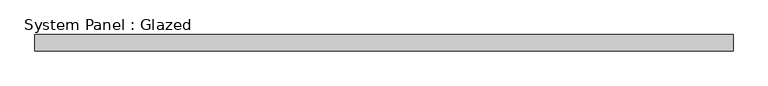
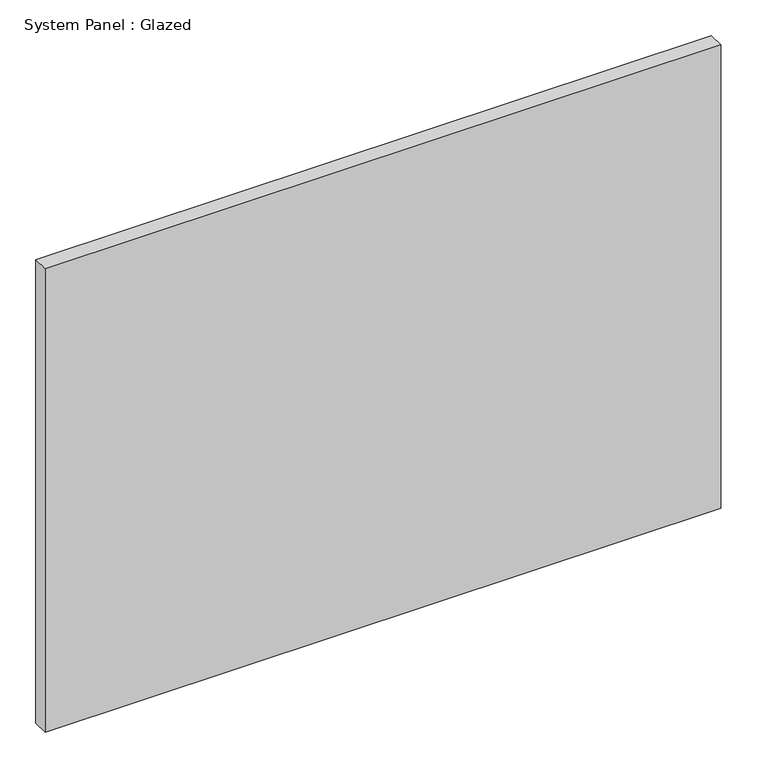
"""IFC4 building model written with IfcOpenShell, lengths in millimetres: plate geometry, System Panel : Glazed."""

from ifc_helpers import new_model, si_unit, origin, origin_with_axes, place, context, project, spatial, polyline, outline, extrude, source, transform, mapped, element, save


def system_panel_glazed_768357cb(model_context):
    return source(origin(), model_context, "Body", "SweptSolid", [
        extrude(outline(polyline([(542.925, 19.05), (-542.925, 19.05), (-542.925, 44.45), (542.925, 44.45), (542.925, 19.05)])), origin_with_axes(), (0.0, 0.0, 1.0), 787.4),
    ])


if __name__ == "__main__":
    model = new_model("IFC4")
    model_context = context("Model", 3, world=origin())
    ifc_project = project(units=[si_unit("LENGTHUNIT", "METRE", prefix="MILLI")], contexts=[model_context])
    site = spatial("IfcSite", under=ifc_project)
    building = spatial("IfcBuilding", under=site)
    placement = place(None, origin())
    system_panel_glazed_shape = system_panel_glazed_768357cb(model_context)
    element("IfcPlate", 1, ObjectType="System Panel : Glazed", at=placement, inside=building, context=model_context, shape_type="MappedRepresentation", body=[
        mapped(system_panel_glazed_shape, transform((0.0, 0.0, 0.0), x_axis=(1.0, 0.0, 0.0), y_axis=(0.0, 1.0, 0.0), z_axis=(0.0, 0.0, 1.0))),
    ])
    save(model, "model.ifc")

# Revit data of these elements
# Type "System Panel : Glazed"
#   Construction Type Id = "GSP4R"
#   Analytic Construction = "1/8 in Pilkington single glazing"
#   Visual Light Transmittance = 0.9
#   Solar Heat Gain Coefficient = 0.86
#   Heat Transfer Coefficient (U) = 1.18115 BTU/(h·ft²·°F)
# Element 1 (IfcPlate, "System Panel : Glazed")
#   Materials on its faces: "Glass"
# Materials
#   "Glass": class "Glass", colour RGB 0 128 192, transparency 0.75, Description = "Soda Lime Glass", Cost = 0
